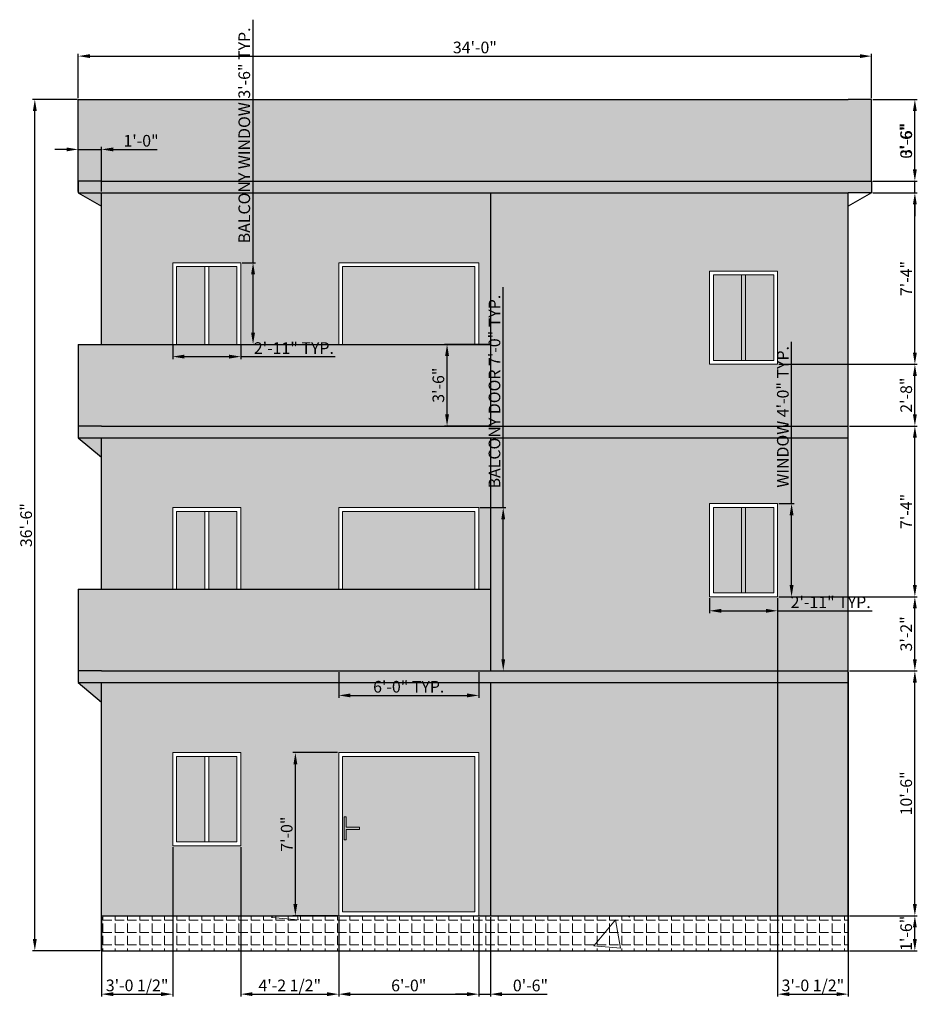
# Model space of a CAD drawing. Units: inches. Extents: x 2129 to 3258, y 1851 to 3021.
# Tile 10 of 10: x 2144 to 2605, y 2514 to 3021. Entities that reach past the tile are written whole.
import ezdxf

# ---------------------------------------------------------------- set-up
doc = ezdxf.new("R2010")
doc.units = ezdxf.units.IN
for name, color, linetype, lineweight in [('A-ANNO-DIMS', 2, 'Continuous', 18), ('A-ELEV', 7, 'Continuous', 25), ('A-ELEV-DOOR', 4, 'Continuous', 18), ('A-ELEV-DOOR-PATT', 34, 'Continuous', 13), ('A-ELEV-GLAZ', 4, 'Continuous', 18), ('A-ELEV-MASN-PATT', 7, 'Continuous', 13)]:
    doc.layers.add(name, color=color, linetype=linetype, lineweight=lineweight)
for name, color, linetype, lineweight, true_color in [('A-ELEV-BASE-PATT', 244, 'Continuous', 13, 0x991b1e), ('A-ELEV-GLAZ-PATT', 143, 'Continuous', 13, 0x7aafdf), ('A-ELEV-HDWR-PATT', 51, 'Continuous', 13, 0xf8f6b0), ('A-ELEV-TRIM-PATT', 244, 'Continuous', 13, 0x991b1e), ('A-ELEV-WALL-PATT', 116, 'Continuous', 13, 0x136734)]:
    doc.layers.add(name, color=color, linetype=linetype, lineweight=lineweight, true_color=true_color)
doc.styles.get("Standard").update_dxf_attribs({"font": 'arial.ttf'})
doc.dimstyles.new('ISO-25', dxfattribs={"dimtxt": 6, "dimasz": 6, "dimexe": 1.25, "dimexo": 0.625, "dimtad": 1, "dimdec": 1, "dimlunit": 3, "dimtxsty": 'Standard', "dimcen": 2.5, "dimclrd": 5, "dimclre": 5, "dimadec": 0, "dimazin": 0, "dimtfac": 1, "dimtdec": 1, "dimtmove": 0, "dimatfit": 3, "dimfxl": 1, "dimarcsym": 0})

# ---------------------------------------------------------------- blocks, each defined once
blk = doc.blocks.new('WIN-ELEV-35X48')
for p, q in [((16.5, 46), (16.5, 2)), ((18.5, 46), (18.5, 2))]:
    blk.add_line(p, q)
for points in [[(0, 0), (35, 0), (35, 48), (0, 48)], [(0, 0), (35, 0), (35, 48), (0, 48)], [(2, 2), (33, 2), (33, 46), (2, 46)]]:
    blk.add_lwpolyline(points, close=True)
blk = doc.blocks.new('WIN-ELEV-BALCONY')
for p, q in [((16.5, 40), (16.5, 0)), ((18.5, 40), (18.5, 0))]:
    blk.add_line(p, q)
for points in [[(35, 0), (35, 42), (0, 42), (0, 0)], [(35, 0), (35, 42), (0, 42), (0, 0)], [(33, 0), (33, 40), (2, 40), (2, 0)]]:
    blk.add_lwpolyline(points)
blk = doc.blocks.new('DOOR-ELEV-BALCONY')
for points in [[(72, 42), (72, 84), (0, 84), (0, 42)], [(72, 42), (72, 84), (0, 84), (0, 42)], [(70, 42), (70, 82), (2, 82), (2, 42)], [(0, 0), (72, 0)], [(0, 0), (72, 0)]]:
    blk.add_lwpolyline(points)
blk = doc.blocks.new('*D80')
at = {"layer": 'A-ANNO-DIMS', "color": 5, "lineweight": -2, "transparency": 16777216}
for p, q in [((2540.83, 2772.1), (2540.83, 2855.28)), ((2534.25, 2772.1), (2542.08, 2772.1)), ((2540.83, 2730.1), (2540.83, 2766.1)), ((2534.25, 2724.1), (2542.08, 2724.1))]:
    blk.add_line(p, q, dxfattribs=at)
at = {"layer": 'A-ANNO-DIMS', "color": 5, "transparency": 16777216}
for points in [[(2539.83, 2766.1), (2541.83, 2766.1), (2540.83, 2772.1)], [(2539.83, 2730.1), (2541.83, 2730.1), (2540.83, 2724.1)]]:
    blk.add_solid(points, dxfattribs=at)
at = {"layer": 'Defpoints', "color": 0, "transparency": 16777216}
for p in [(2533.63, 2772.1), (2540.83, 2772.1), (2533.63, 2724.1)]:
    blk.add_point(p, dxfattribs=at)
at = {"layer": 'A-ANNO-DIMS', "color": 0, "transparency": 16777216, "insert": (2537.1, 2816.69), "char_height": 6, "attachment_point": 5, "rotation": 90}
blk.add_mtext('WINDOW 4\'-0" TYP.', dxfattribs=at)
blk = doc.blocks.new('*D81')
at = {"layer": 'A-ANNO-DIMS', "color": 5, "lineweight": -2, "transparency": 16777216}
for p, q in [((2498.63, 2723.48), (2498.63, 2715.65)), ((2533.63, 2723.48), (2533.63, 2715.65)), ((2504.63, 2716.9), (2527.63, 2716.9)), ((2533.63, 2716.9), (2582.21, 2716.9))]:
    blk.add_line(p, q, dxfattribs=at)
at = {"layer": 'A-ANNO-DIMS', "color": 5, "transparency": 16777216}
for points in [[(2504.63, 2717.9), (2504.63, 2715.9), (2498.63, 2716.9)], [(2527.63, 2717.9), (2527.63, 2715.9), (2533.63, 2716.9)]]:
    blk.add_solid(points, dxfattribs=at)
at = {"layer": 'Defpoints', "color": 0, "transparency": 16777216}
for p in [(2498.63, 2724.1), (2533.63, 2724.1), (2533.63, 2716.9)]:
    blk.add_point(p, dxfattribs=at)
at = {"layer": 'A-ANNO-DIMS', "color": 0, "transparency": 16777216, "insert": (2560.92, 2720.54), "char_height": 6, "attachment_point": 5}
blk.add_mtext('2\'-11" TYP.', dxfattribs=at)
blk = doc.blocks.new('*D82')
at = {"layer": 'A-ANNO-DIMS', "color": 5, "lineweight": -2, "transparency": 16777216}
for p, q in [((2263.86, 2895.97), (2263.86, 3021.02)), ((2258.19, 2895.97), (2265.11, 2895.97)), ((2263.86, 2859.97), (2263.86, 2889.97)), ((2258.19, 2853.97), (2265.11, 2853.97))]:
    blk.add_line(p, q, dxfattribs=at)
at = {"layer": 'A-ANNO-DIMS', "color": 5, "transparency": 16777216}
for points in [[(2262.86, 2889.97), (2264.86, 2889.97), (2263.86, 2895.97)], [(2262.86, 2859.97), (2264.86, 2859.97), (2263.86, 2853.97)]]:
    blk.add_solid(points, dxfattribs=at)
at = {"layer": 'Defpoints', "color": 0, "transparency": 16777216}
for p in [(2257.56, 2895.97), (2263.86, 2895.97), (2257.56, 2853.97)]:
    blk.add_point(p, dxfattribs=at)
at = {"layer": 'A-ANNO-DIMS', "color": 0, "transparency": 16777216, "insert": (2260.13, 2961.49), "char_height": 6, "attachment_point": 5, "rotation": 90}
blk.add_mtext('BALCONY WINDOW 3\'-6" TYP.', dxfattribs=at)
blk = doc.blocks.new('*D83')
at = {"layer": 'A-ANNO-DIMS', "color": 5, "lineweight": -2, "transparency": 16777216}
for p, q in [((2222.56, 2853.34), (2222.56, 2846.42)), ((2257.56, 2853.34), (2257.56, 2846.42)), ((2228.56, 2847.67), (2251.56, 2847.67)), ((2257.56, 2847.67), (2306.15, 2847.67))]:
    blk.add_line(p, q, dxfattribs=at)
at = {"layer": 'A-ANNO-DIMS', "color": 5, "transparency": 16777216}
for points in [[(2228.56, 2848.67), (2228.56, 2846.67), (2222.56, 2847.67)], [(2251.56, 2848.67), (2251.56, 2846.67), (2257.56, 2847.67)]]:
    blk.add_solid(points, dxfattribs=at)
at = {"layer": 'Defpoints', "color": 0, "transparency": 16777216}
for p in [(2222.56, 2853.97), (2257.56, 2853.97), (2257.56, 2847.67)]:
    blk.add_point(p, dxfattribs=at)
at = {"layer": 'A-ANNO-DIMS', "color": 0, "transparency": 16777216, "insert": (2284.86, 2851.3), "char_height": 6, "attachment_point": 5}
blk.add_mtext('2\'-11" TYP.', dxfattribs=at)
blk = doc.blocks.new('*D84')
at = {"layer": 'A-ANNO-DIMS', "color": 5, "lineweight": -2, "transparency": 16777216}
for p, q in [((2392.53, 2769.97), (2392.53, 2883.39)), ((2380.55, 2769.97), (2393.78, 2769.97)), ((2392.53, 2691.97), (2392.53, 2763.97)), ((2380.55, 2685.97), (2393.78, 2685.97))]:
    blk.add_line(p, q, dxfattribs=at)
at = {"layer": 'A-ANNO-DIMS', "color": 5, "transparency": 16777216}
for points in [[(2391.53, 2763.97), (2393.53, 2763.97), (2392.53, 2769.97)], [(2391.53, 2691.97), (2393.53, 2691.97), (2392.53, 2685.97)]]:
    blk.add_solid(points, dxfattribs=at)
at = {"layer": 'Defpoints', "color": 0, "transparency": 16777216}
for p in [(2379.93, 2769.97), (2392.53, 2769.97), (2379.93, 2685.97)]:
    blk.add_point(p, dxfattribs=at)
at = {"layer": 'A-ANNO-DIMS', "color": 0, "transparency": 16777216, "insert": (2388.8, 2829.68), "char_height": 6, "attachment_point": 5, "rotation": 90}
blk.add_mtext('BALCONY DOOR 7\'-0" TYP.', dxfattribs=at)
blk = doc.blocks.new('*D85')
at = {"layer": 'A-ANNO-DIMS', "color": 5, "lineweight": -2, "transparency": 16777216}
for p, q in [((2307.93, 2685.34), (2307.93, 2672.12)), ((2379.93, 2685.34), (2379.93, 2672.12)), ((2313.93, 2673.37), (2373.93, 2673.37))]:
    blk.add_line(p, q, dxfattribs=at)
at = {"layer": 'A-ANNO-DIMS', "color": 5, "transparency": 16777216}
for points in [[(2313.93, 2674.37), (2313.93, 2672.37), (2307.93, 2673.37)], [(2373.93, 2674.37), (2373.93, 2672.37), (2379.93, 2673.37)]]:
    blk.add_solid(points, dxfattribs=at)
at = {"layer": 'Defpoints', "color": 0, "transparency": 16777216}
for p in [(2307.93, 2685.97), (2379.93, 2685.97), (2379.93, 2673.37)]:
    blk.add_point(p, dxfattribs=at)
at = {"layer": 'A-ANNO-DIMS', "color": 0, "transparency": 16777216, "insert": (2343.93, 2677.05), "char_height": 6, "attachment_point": 5}
blk.add_mtext('6\'-0" TYP.', dxfattribs=at)
blk = doc.blocks.new('*D115')
at = {"layer": 'A-ANNO-DIMS', "color": 5, "lineweight": -2, "transparency": 16777216}
for p, q in [((2173.98, 2980.59), (2173.98, 3003.52)), ((2179.98, 3002.27), (2575.93, 3002.27)), ((2581.93, 2980.59), (2581.93, 3003.52))]:
    blk.add_line(p, q, dxfattribs=at)
at = {"layer": 'A-ANNO-DIMS', "color": 5, "transparency": 16777216}
for points in [[(2179.98, 3003.27), (2179.98, 3001.27), (2173.98, 3002.27)], [(2575.93, 3003.27), (2575.93, 3001.27), (2581.93, 3002.27)]]:
    blk.add_solid(points, dxfattribs=at)
at = {"layer": 'Defpoints', "color": 0, "transparency": 16777216}
for p in [(2581.93, 3002.27), (2173.98, 2979.97), (2581.93, 2979.97)]:
    blk.add_point(p, dxfattribs=at)
at = {"layer": 'A-ANNO-DIMS', "color": 0, "transparency": 16777216, "insert": (2377.95, 3005.96), "char_height": 6, "attachment_point": 5}
blk.add_mtext('34\'-0"', dxfattribs=at)
blk = doc.blocks.new('*D116')
at = {"layer": 'A-ANNO-DIMS', "color": 5, "lineweight": -2, "transparency": 16777216}
for p, q in [((2173.35, 2979.97), (2150.38, 2979.97)), ((2151.63, 2547.97), (2151.63, 2973.97)), ((2185.3, 2541.97), (2150.38, 2541.97))]:
    blk.add_line(p, q, dxfattribs=at)
at = {"layer": 'A-ANNO-DIMS', "color": 5, "transparency": 16777216}
for points in [[(2150.63, 2973.97), (2152.63, 2973.97), (2151.63, 2979.97)], [(2150.63, 2547.97), (2152.63, 2547.97), (2151.63, 2541.97)]]:
    blk.add_solid(points, dxfattribs=at)
at = {"layer": 'Defpoints', "color": 0, "transparency": 16777216}
for p in [(2151.63, 2979.97), (2173.98, 2979.97), (2185.93, 2541.97)]:
    blk.add_point(p, dxfattribs=at)
at = {"layer": 'A-ANNO-DIMS', "color": 0, "transparency": 16777216, "insert": (2147.94, 2760.97), "char_height": 6, "attachment_point": 5, "rotation": 90}
blk.add_mtext('36\'-6"', dxfattribs=at)
blk = doc.blocks.new('*D117')
at = {"layer": 'A-ANNO-DIMS', "color": 5, "lineweight": -2, "transparency": 16777216}
for p, q in [((2570.55, 2559.97), (2605.48, 2559.97)), ((2604.23, 2547.97), (2604.23, 2553.97)), ((2570.55, 2541.97), (2605.48, 2541.97))]:
    blk.add_line(p, q, dxfattribs=at)
at = {"layer": 'A-ANNO-DIMS', "color": 5, "transparency": 16777216}
for points in [[(2603.23, 2553.97), (2605.23, 2553.97), (2604.23, 2559.97)], [(2603.23, 2547.97), (2605.23, 2547.97), (2604.23, 2541.97)]]:
    blk.add_solid(points, dxfattribs=at)
at = {"layer": 'Defpoints', "color": 0, "transparency": 16777216}
for p in [(2569.93, 2559.97), (2604.23, 2559.97), (2569.93, 2541.97)]:
    blk.add_point(p, dxfattribs=at)
at = {"layer": 'A-ANNO-DIMS', "color": 0, "transparency": 16777216, "insert": (2600.54, 2550.97), "char_height": 6, "attachment_point": 5, "rotation": 90}
blk.add_mtext('1\'-6"', dxfattribs=at)
blk = doc.blocks.new('*D118')
at = {"layer": 'A-ANNO-DIMS', "color": 5, "lineweight": -2, "transparency": 16777216}
for p, q in [((2570.55, 2685.97), (2605.48, 2685.97)), ((2604.23, 2565.97), (2604.23, 2679.97)), ((2570.55, 2559.97), (2605.48, 2559.97))]:
    blk.add_line(p, q, dxfattribs=at)
at = {"layer": 'A-ANNO-DIMS', "color": 5, "transparency": 16777216}
for points in [[(2603.23, 2679.97), (2605.23, 2679.97), (2604.23, 2685.97)], [(2603.23, 2565.97), (2605.23, 2565.97), (2604.23, 2559.97)]]:
    blk.add_solid(points, dxfattribs=at)
at = {"layer": 'Defpoints', "color": 0, "transparency": 16777216}
for p in [(2569.93, 2685.97), (2604.23, 2685.97), (2569.93, 2559.97)]:
    blk.add_point(p, dxfattribs=at)
at = {"layer": 'A-ANNO-DIMS', "color": 0, "transparency": 16777216, "insert": (2600.54, 2622.97), "char_height": 6, "attachment_point": 5, "rotation": 90}
blk.add_mtext('10\'-6"', dxfattribs=at)
blk = doc.blocks.new('*D119')
at = {"layer": 'A-ANNO-DIMS', "color": 5, "lineweight": -2, "transparency": 16777216}
for p, q in [((2534.25, 2724.1), (2605.48, 2724.1)), ((2604.23, 2691.97), (2604.23, 2718.1)), ((2570.55, 2685.97), (2605.48, 2685.97))]:
    blk.add_line(p, q, dxfattribs=at)
at = {"layer": 'A-ANNO-DIMS', "color": 5, "transparency": 16777216}
for points in [[(2603.23, 2718.1), (2605.23, 2718.1), (2604.23, 2724.1)], [(2603.23, 2691.97), (2605.23, 2691.97), (2604.23, 2685.97)]]:
    blk.add_solid(points, dxfattribs=at)
at = {"layer": 'Defpoints', "color": 0, "transparency": 16777216}
for p in [(2533.63, 2724.1), (2604.23, 2724.1), (2569.93, 2685.97)]:
    blk.add_point(p, dxfattribs=at)
at = {"layer": 'A-ANNO-DIMS', "color": 0, "transparency": 16777216, "insert": (2600.54, 2705.03), "char_height": 6, "attachment_point": 5, "rotation": 90}
blk.add_mtext('3\'-2"', dxfattribs=at)
blk = doc.blocks.new('*D120')
at = {"layer": 'A-ANNO-DIMS', "color": 5, "lineweight": -2, "transparency": 16777216}
for p, q in [((2570.552986, 2811.965219), (2605.477986, 2811.965219)), ((2604.227986, 2730.103007), (2604.227986, 2805.965219)), ((2534.252329, 2724.103007), (2605.477986, 2724.103007))]:
    blk.add_line(p, q, dxfattribs=at)
at = {"layer": 'A-ANNO-DIMS', "color": 5, "transparency": 16777216}
for points in [[(2603.227986, 2805.965219), (2605.227986, 2805.965219), (2604.227986, 2811.965219)], [(2603.227986, 2730.103007), (2605.227986, 2730.103007), (2604.227986, 2724.103007)]]:
    blk.add_solid(points, dxfattribs=at)
at = {"layer": 'Defpoints', "color": 0, "transparency": 16777216}
for p in [(2569.927986, 2811.965219), (2604.227986, 2811.965219), (2533.627329, 2724.103007)]:
    blk.add_point(p, dxfattribs=at)
at = {"layer": 'A-ANNO-DIMS', "color": 0, "transparency": 16777216, "insert": (2600.602986, 2768.034113), "char_height": 6, "attachment_point": 5, "rotation": 90}
blk.add_mtext('7\'-4"', dxfattribs=at)
blk = doc.blocks.new('*D121')
at = {"layer": 'A-ANNO-DIMS', "color": 5, "lineweight": -2, "transparency": 16777216}
for p, q in [((2534.25, 2843.72), (2605.48, 2843.72)), ((2604.23, 2817.97), (2604.23, 2837.72)), ((2570.55, 2811.97), (2605.48, 2811.97))]:
    blk.add_line(p, q, dxfattribs=at)
at = {"layer": 'A-ANNO-DIMS', "color": 5, "transparency": 16777216}
for points in [[(2603.23, 2837.72), (2605.23, 2837.72), (2604.23, 2843.72)], [(2603.23, 2817.97), (2605.23, 2817.97), (2604.23, 2811.97)]]:
    blk.add_solid(points, dxfattribs=at)
at = {"layer": 'Defpoints', "color": 0, "transparency": 16777216}
for p in [(2533.63, 2843.72), (2604.23, 2843.72), (2569.93, 2811.97)]:
    blk.add_point(p, dxfattribs=at)
at = {"layer": 'A-ANNO-DIMS', "color": 0, "transparency": 16777216, "insert": (2600.54, 2827.84), "char_height": 6, "attachment_point": 5, "rotation": 90}
blk.add_mtext('2\'-8"', dxfattribs=at)
blk = doc.blocks.new('*D122')
at = {"layer": 'A-ANNO-DIMS', "color": 5, "lineweight": -2, "transparency": 16777216}
for p, q in [((2582.552986, 2931.965219), (2605.477986, 2931.965219)), ((2604.227986, 2849.721947), (2604.227986, 2925.965219)), ((2534.252329, 2843.721947), (2605.477986, 2843.721947))]:
    blk.add_line(p, q, dxfattribs=at)
at = {"layer": 'A-ANNO-DIMS', "color": 5, "transparency": 16777216}
for points in [[(2603.227986, 2925.965219), (2605.227986, 2925.965219), (2604.227986, 2931.965219)], [(2603.227986, 2849.721947), (2605.227986, 2849.721947), (2604.227986, 2843.721947)]]:
    blk.add_solid(points, dxfattribs=at)
at = {"layer": 'Defpoints', "color": 0, "transparency": 16777216}
for p in [(2581.927986, 2931.965219), (2604.227986, 2931.965219), (2533.627329, 2843.721947)]:
    blk.add_point(p, dxfattribs=at)
at = {"layer": 'A-ANNO-DIMS', "color": 0, "transparency": 16777216, "insert": (2600.602986, 2887.843583), "char_height": 6, "attachment_point": 5, "rotation": 90}
blk.add_mtext('7\'-4"', dxfattribs=at)
blk = doc.blocks.new('*D123')
at = {"layer": 'A-ANNO-DIMS', "color": 5, "lineweight": -2, "transparency": 16777216}
for p, q in [((2604.23, 2943.97), (2604.23, 2967.16)), ((2582.55, 2937.97), (2605.48, 2937.97)), ((2604.23, 2931.97), (2604.23, 2937.97)), ((2582.55, 2931.97), (2605.48, 2931.97)), ((2604.23, 2925.97), (2604.23, 2919.97))]:
    blk.add_line(p, q, dxfattribs=at)
at = {"layer": 'A-ANNO-DIMS', "color": 5, "transparency": 16777216}
for points in [[(2603.23, 2943.97), (2605.23, 2943.97), (2604.23, 2937.97)], [(2603.23, 2925.97), (2605.23, 2925.97), (2604.23, 2931.97)]]:
    blk.add_solid(points, dxfattribs=at)
at = {"layer": 'Defpoints', "color": 0, "transparency": 16777216}
for p in [(2581.93, 2937.97), (2604.23, 2937.97), (2581.93, 2931.97)]:
    blk.add_point(p, dxfattribs=at)
at = {"layer": 'A-ANNO-DIMS', "color": 0, "transparency": 16777216, "insert": (2600.54, 2958.56), "char_height": 6, "attachment_point": 5, "rotation": 90}
blk.add_mtext('0\'-6"', dxfattribs=at)
blk = doc.blocks.new('*D124')
at = {"layer": 'A-ANNO-DIMS', "color": 5, "lineweight": -2, "transparency": 16777216}
for p, q in [((2582.55, 2979.97), (2605.48, 2979.97)), ((2604.23, 2943.97), (2604.23, 2973.97)), ((2582.55, 2937.97), (2605.48, 2937.97))]:
    blk.add_line(p, q, dxfattribs=at)
at = {"layer": 'A-ANNO-DIMS', "color": 5, "transparency": 16777216}
for points in [[(2603.23, 2973.97), (2605.23, 2973.97), (2604.23, 2979.97)], [(2603.23, 2943.97), (2605.23, 2943.97), (2604.23, 2937.97)]]:
    blk.add_solid(points, dxfattribs=at)
at = {"layer": 'Defpoints', "color": 0, "transparency": 16777216}
for p in [(2581.93, 2979.97), (2604.23, 2979.97), (2581.93, 2937.97)]:
    blk.add_point(p, dxfattribs=at)
at = {"layer": 'A-ANNO-DIMS', "color": 0, "transparency": 16777216, "insert": (2600.54, 2958.97), "char_height": 6, "attachment_point": 5, "rotation": 90}
blk.add_mtext('3\'-6"', dxfattribs=at)
blk = doc.blocks.new('*D125')
at = {"layer": 'A-ANNO-DIMS', "color": 5, "lineweight": -2, "transparency": 16777216}
for p, q in [((2222.56, 2595.34), (2222.56, 2518.42)), ((2185.93, 2559.34), (2185.93, 2518.42)), ((2191.93, 2519.67), (2216.56, 2519.67))]:
    blk.add_line(p, q, dxfattribs=at)
at = {"layer": 'A-ANNO-DIMS', "color": 5, "transparency": 16777216}
for points in [[(2191.93, 2520.67), (2191.93, 2518.67), (2185.93, 2519.67)], [(2216.56, 2520.67), (2216.56, 2518.67), (2222.56, 2519.67)]]:
    blk.add_solid(points, dxfattribs=at)
at = {"layer": 'Defpoints', "color": 0, "transparency": 16777216}
for p in [(2222.56, 2595.97), (2185.93, 2559.97), (2222.56, 2519.67)]:
    blk.add_point(p, dxfattribs=at)
at = {"layer": 'A-ANNO-DIMS', "color": 0, "transparency": 16777216, "insert": (2204.25, 2523.39), "char_height": 6, "attachment_point": 5}
blk.add_mtext('3\'-0 1/2"', dxfattribs=at)
blk = doc.blocks.new('*D126')
at = {"layer": 'A-ANNO-DIMS', "color": 5, "lineweight": -2, "transparency": 16777216}
for p, q in [((2257.56, 2595.34), (2257.56, 2518.42)), ((2307.93, 2559.34), (2307.93, 2518.42)), ((2263.56, 2519.67), (2301.93, 2519.67))]:
    blk.add_line(p, q, dxfattribs=at)
at = {"layer": 'A-ANNO-DIMS', "color": 5, "transparency": 16777216}
for points in [[(2263.56, 2520.67), (2263.56, 2518.67), (2257.56, 2519.67)], [(2301.93, 2520.67), (2301.93, 2518.67), (2307.93, 2519.67)]]:
    blk.add_solid(points, dxfattribs=at)
at = {"layer": 'Defpoints', "color": 0, "transparency": 16777216}
for p in [(2257.56, 2595.97), (2307.93, 2559.97), (2307.93, 2519.67)]:
    blk.add_point(p, dxfattribs=at)
at = {"layer": 'A-ANNO-DIMS', "color": 0, "transparency": 16777216, "insert": (2282.75, 2523.39), "char_height": 6, "attachment_point": 5}
blk.add_mtext('4\'-2 1/2"', dxfattribs=at)
blk = doc.blocks.new('*D127')
at = {"layer": 'A-ANNO-DIMS', "color": 5, "lineweight": -2, "transparency": 16777216}
for p, q in [((2379.93, 2559.34), (2379.93, 2518.42)), ((2385.93, 2559.34), (2385.93, 2518.42)), ((2373.93, 2519.67), (2367.93, 2519.67)), ((2379.93, 2519.67), (2385.93, 2519.67)), ((2391.93, 2519.67), (2415.13, 2519.67))]:
    blk.add_line(p, q, dxfattribs=at)
at = {"layer": 'A-ANNO-DIMS', "color": 5, "transparency": 16777216}
for points in [[(2373.93, 2520.67), (2373.93, 2518.67), (2379.93, 2519.67)], [(2391.93, 2520.67), (2391.93, 2518.67), (2385.93, 2519.67)]]:
    blk.add_solid(points, dxfattribs=at)
at = {"layer": 'Defpoints', "color": 0, "transparency": 16777216}
for p in [(2379.93, 2559.97), (2385.93, 2559.97), (2385.93, 2519.67)]:
    blk.add_point(p, dxfattribs=at)
at = {"layer": 'A-ANNO-DIMS', "color": 0, "transparency": 16777216, "insert": (2406.53, 2523.35), "char_height": 6, "attachment_point": 5}
blk.add_mtext('0\'-6"', dxfattribs=at)
blk = doc.blocks.new('*D128')
at = {"layer": 'A-ANNO-DIMS', "color": 5, "lineweight": -2, "transparency": 16777216}
for p, q in [((2533.63, 2723.48), (2533.63, 2518.42)), ((2569.93, 2685.34), (2569.93, 2518.42)), ((2539.63, 2519.67), (2563.93, 2519.67))]:
    blk.add_line(p, q, dxfattribs=at)
at = {"layer": 'A-ANNO-DIMS', "color": 5, "transparency": 16777216}
for points in [[(2539.63, 2520.67), (2539.63, 2518.67), (2533.63, 2519.67)], [(2563.93, 2520.67), (2563.93, 2518.67), (2569.93, 2519.67)]]:
    blk.add_solid(points, dxfattribs=at)
at = {"layer": 'Defpoints', "color": 0, "transparency": 16777216}
for p in [(2533.63, 2724.1), (2569.93, 2685.97), (2569.93, 2519.67)]:
    blk.add_point(p, dxfattribs=at)
at = {"layer": 'A-ANNO-DIMS', "color": 0, "transparency": 16777216, "insert": (2551.78, 2523.39), "char_height": 6, "attachment_point": 5}
blk.add_mtext('3\'-0 1/2"', dxfattribs=at)
blk = doc.blocks.new('*D129')
at = {"layer": 'A-ANNO-DIMS', "color": 5, "lineweight": -2, "transparency": 16777216}
for p, q in [((2307.3, 2643.97), (2284.38, 2643.97)), ((2285.63, 2565.97), (2285.63, 2637.97)), ((2307.3, 2559.97), (2284.38, 2559.97))]:
    blk.add_line(p, q, dxfattribs=at)
at = {"layer": 'A-ANNO-DIMS', "color": 5, "transparency": 16777216}
for points in [[(2284.63, 2637.97), (2286.63, 2637.97), (2285.63, 2643.97)], [(2284.63, 2565.97), (2286.63, 2565.97), (2285.63, 2559.97)]]:
    blk.add_solid(points, dxfattribs=at)
at = {"layer": 'Defpoints', "color": 0, "transparency": 16777216}
for p in [(2285.63, 2643.97), (2307.93, 2643.97), (2307.93, 2559.97)]:
    blk.add_point(p, dxfattribs=at)
at = {"layer": 'A-ANNO-DIMS', "color": 0, "transparency": 16777216, "insert": (2281.94, 2601.97), "char_height": 6, "attachment_point": 5, "rotation": 90}
blk.add_mtext('7\'-0"', dxfattribs=at)
blk = doc.blocks.new('*D130')
at = {"layer": 'A-ANNO-DIMS', "color": 5, "lineweight": -2, "transparency": 16777216}
for p, q in [((2385.3, 2853.97), (2362.38, 2853.97)), ((2363.63, 2817.97), (2363.63, 2847.97)), ((2385.3, 2811.97), (2362.38, 2811.97))]:
    blk.add_line(p, q, dxfattribs=at)
at = {"layer": 'A-ANNO-DIMS', "color": 5, "transparency": 16777216}
for points in [[(2362.63, 2847.97), (2364.63, 2847.97), (2363.63, 2853.97)], [(2362.63, 2817.97), (2364.63, 2817.97), (2363.63, 2811.97)]]:
    blk.add_solid(points, dxfattribs=at)
at = {"layer": 'Defpoints', "color": 0, "transparency": 16777216}
for p in [(2363.63, 2853.97), (2385.93, 2853.97), (2385.93, 2811.97)]:
    blk.add_point(p, dxfattribs=at)
at = {"layer": 'A-ANNO-DIMS', "color": 0, "transparency": 16777216, "insert": (2359.94, 2832.97), "char_height": 6, "attachment_point": 5, "rotation": 90}
blk.add_mtext('3\'-6"', dxfattribs=at)
blk = doc.blocks.new('*D131')
at = {"layer": 'A-ANNO-DIMS', "color": 5, "lineweight": -2, "transparency": 16777216}
for p, q in [((2307.93, 2559.34), (2307.93, 2518.42)), ((2379.93, 2559.34), (2379.93, 2518.42)), ((2313.93, 2519.67), (2373.93, 2519.67))]:
    blk.add_line(p, q, dxfattribs=at)
at = {"layer": 'A-ANNO-DIMS', "color": 5, "transparency": 16777216}
for points in [[(2313.93, 2520.67), (2313.93, 2518.67), (2307.93, 2519.67)], [(2373.93, 2520.67), (2373.93, 2518.67), (2379.93, 2519.67)]]:
    blk.add_solid(points, dxfattribs=at)
at = {"layer": 'Defpoints', "color": 0, "transparency": 16777216}
for p in [(2307.93, 2559.97), (2379.93, 2559.97), (2379.93, 2519.67)]:
    blk.add_point(p, dxfattribs=at)
at = {"layer": 'A-ANNO-DIMS', "color": 0, "transparency": 16777216, "insert": (2343.93, 2523.35), "char_height": 6, "attachment_point": 5}
blk.add_mtext('6\'-0"', dxfattribs=at)
blk = doc.blocks.new('*D132')
at = {"layer": 'A-ANNO-DIMS', "color": 5, "lineweight": -2, "transparency": 16777216}
for p, q in [((2167.93, 2954.27), (2161.93, 2954.27)), ((2173.93, 2932.59), (2173.93, 2955.52)), ((2173.93, 2954.27), (2185.93, 2954.27)), ((2185.93, 2932.59), (2185.93, 2955.52)), ((2191.93, 2954.27), (2214.56, 2954.27))]:
    blk.add_line(p, q, dxfattribs=at)
at = {"layer": 'A-ANNO-DIMS', "color": 5, "transparency": 16777216}
for points in [[(2167.93, 2955.27), (2167.93, 2953.27), (2173.93, 2954.27)], [(2191.93, 2955.27), (2191.93, 2953.27), (2185.93, 2954.27)]]:
    blk.add_solid(points, dxfattribs=at)
at = {"layer": 'Defpoints', "color": 0, "transparency": 16777216}
for p in [(2185.93, 2954.27), (2173.93, 2931.97), (2185.93, 2931.97)]:
    blk.add_point(p, dxfattribs=at)
at = {"layer": 'A-ANNO-DIMS', "color": 0, "transparency": 16777216, "insert": (2206.25, 2957.95), "char_height": 6, "attachment_point": 5}
blk.add_mtext('1\'-0"', dxfattribs=at)

msp = doc.modelspace()

# ---------------------------------------------------------------- hatches: boundary and pattern name
at = {"layer": 'A-ELEV-BASE-PATT', "transparency": 33554585}
h = msp.add_hatch(dxfattribs=at)
h.set_pattern_fill('AR-CONC', color=256, scale=0.91)
h.set_pattern_definition([(50, (0, -150.12), (165.788, -14.5046), [17.3355, -190.6905]), (355, (0, -150.12), (-32.0715, 173.862), [13.8684, -152.553]), (100.4514, (13.82, -151.33), (133.7165, 159.357), [14.733, -162.062]), (46.184, (0, -103.9), (246.682, -38.259), [26.003, -286.036]), (96.6356, (20.56, -107.08), (216.038, 225.158), [22.1, -243.093]), (351.184, (0, -103.9), (216.038, 225.158), [20.803, -228.828]), (21, (23.11, -115.45), (137.969, -93.0613), [17.3355, -190.6905]), (326, (23.11, -115.45), (56.24, 167.611), [13.8684, -152.5524]), (71.4514, (34.61, -123.21), (194.209, 74.55), [14.733, -162.062]), (37.5, (0, -150.125), (2.8106, 76.9451), [0, -150.7033, 0, -154.8638, 0, -153.1302]), (7.5, (0, -150.125), (60.8059, 91.1643), [0, -88.2955, 0, -147.2362, 0, -58.3629]), (327.5, (-51.544, -150.125), (123.3874, -5.2132), [0, -57.785, 0, -180.2892, 0, -239.23]), (317.5, (-74.66, -150.12), (134.7976, 23.138), [0, -75.1205, 0, -119.7305, 0, -169.888])])
h.paths.add_polyline_path([(2569.93, 2559.97), (2185.93, 2559.97), (2185.93, 2541.97), (2569.93, 2541.97)])
at = {"layer": 'A-ELEV-DOOR-PATT', "transparency": 33554658}
h = msp.add_hatch(color=256, dxfattribs=at)
h.dxf.hatch_style = 1
h.paths.add_polyline_path([(2377.93, 2767.97), (2309.93, 2767.97), (2309.93, 2727.97), (2377.93, 2727.97)])
h.paths.add_polyline_path([(2377.93, 2893.97), (2309.93, 2893.97), (2309.93, 2853.97), (2377.93, 2853.97)])
h = msp.add_hatch(color=256, dxfattribs=at)
h.dxf.hatch_style = 1
h.paths.add_polyline_path([(2377.93, 2641.97), (2309.93, 2641.97), (2309.93, 2561.97), (2377.93, 2561.97)])
at = {"layer": 'A-ELEV-GLAZ-PATT', "transparency": 33554658}
h = msp.add_hatch(color=256, dxfattribs=at)
h.dxf.hatch_style = 1
h.paths.add_polyline_path([(2239.06, 2641.97), (2224.56, 2641.97), (2224.56, 2597.97), (2239.06, 2597.97)])
h.paths.add_polyline_path([(2255.56, 2641.97), (2241.06, 2641.97), (2241.06, 2597.97), (2255.56, 2597.97)])
h.paths.add_polyline_path([(2239.06, 2767.97), (2224.56, 2767.97), (2224.56, 2727.97), (2239.06, 2727.97)])
h.paths.add_polyline_path([(2255.56, 2767.97), (2241.06, 2767.97), (2241.06, 2727.97), (2255.56, 2727.97)])
h.paths.add_polyline_path([(2239.06, 2893.97), (2224.56, 2893.97), (2224.56, 2853.97), (2239.06, 2853.97)])
h.paths.add_polyline_path([(2255.56, 2893.97), (2241.06, 2893.97), (2241.06, 2853.97), (2255.56, 2853.97)])
h.paths.add_polyline_path([(2515.13, 2889.72), (2500.63, 2889.72), (2500.63, 2845.72), (2515.13, 2845.72)])
h.paths.add_polyline_path([(2531.63, 2889.72), (2515.13, 2889.72), (2515.13, 2845.72), (2531.63, 2845.72)])
h.paths.add_polyline_path([(2515.13, 2770.1), (2500.63, 2770.1), (2500.63, 2726.1), (2515.13, 2726.1)])
h.paths.add_polyline_path([(2531.63, 2770.1), (2515.13, 2770.1), (2515.13, 2726.1), (2531.63, 2726.1)])
at = {"layer": 'A-ELEV-HDWR-PATT', "transparency": 33554585}
h = msp.add_hatch(color=256, dxfattribs=at)
h.dxf.hatch_style = 1
h.paths.add_polyline_path([(2311.75, 2604.38), (2318.56, 2604.38), (2318.56, 2605.59), (2311.75, 2605.59), (2311.75, 2610.87), (2310.78, 2610.87), (2310.78, 2598.98), (2311.75, 2598.98)])
at = {"layer": 'A-ELEV-MASN-PATT', "transparency": 33554585}
h = msp.add_hatch(dxfattribs=at)
h.set_pattern_fill('ANGLE', color=256, scale=0.91)
h.set_pattern_definition([(0, (0, -150.1245), (0, 6.35635), [4.6228, -1.73355]), (90, (0, -150.1245), (-6.35635, 4e-16), [4.6228, -1.73355])])
h.paths.add_polyline_path([(2569.93, 2559.97), (2185.93, 2559.97), (2185.93, 2541.97), (2569.93, 2541.97)])
at = {"layer": 'A-ELEV-TRIM-PATT', "transparency": 33554585}
h = msp.add_hatch(color=256, dxfattribs=at)
h.dxf.hatch_style = 1
h.paths.add_polyline_path([(2581.93, 2979.97), (2569.93, 2979.97), (2185.93, 2979.97), (2173.98, 2979.97), (2173.98, 2937.97), (2185.93, 2937.97), (2569.93, 2937.97), (2581.93, 2937.97)])
h = msp.add_hatch(color=256, dxfattribs=at)
h.dxf.hatch_style = 1
h.paths.add_polyline_path([(2581.93, 2937.97), (2569.93, 2937.97), (2185.93, 2937.97), (2173.93, 2937.97), (2173.93, 2931.97), (2185.93, 2931.97), (2569.93, 2931.97), (2581.93, 2931.97)])
h = msp.add_hatch(color=256, dxfattribs=at)
h.dxf.hatch_style = 1
h.paths.add_polyline_path([(2185.93, 2931.97), (2173.93, 2931.97), (2185.93, 2925.04)])
h = msp.add_hatch(color=256, dxfattribs=at)
h.dxf.hatch_style = 1
h.paths.add_polyline_path([(2385.93, 2853.97), (2173.93, 2853.97), (2173.93, 2811.97), (2185.93, 2811.97), (2385.93, 2811.97)])
h.paths.add_polyline_path([(2385.93, 2727.97), (2173.93, 2727.97), (2173.93, 2685.97), (2185.93, 2685.97), (2385.93, 2685.97)])
h = msp.add_hatch(color=256, dxfattribs=at)
h.dxf.hatch_style = 1
h.paths.add_polyline_path([(2569.93, 2811.97), (2185.93, 2811.97), (2173.93, 2811.97), (2173.93, 2805.97), (2185.93, 2805.97), (2569.93, 2805.97)])
h.paths.add_polyline_path([(2185.93, 2805.97), (2173.93, 2805.97), (2185.93, 2795.9)])
h.paths.add_polyline_path([(2569.93, 2685.97), (2185.93, 2685.97), (2173.93, 2685.97), (2173.93, 2679.97), (2185.93, 2679.97), (2569.93, 2679.97)])
h.paths.add_polyline_path([(2185.93, 2679.97), (2173.93, 2679.97), (2185.93, 2669.9)])
at = {"layer": 'A-ELEV-WALL-PATT', "transparency": 33554585}
h = msp.add_hatch(color=256, dxfattribs=at)
h.dxf.hatch_style = 1
h.paths.add_polyline_path([(2385.93, 2931.97), (2185.93, 2931.97), (2185.93, 2853.97), (2222.56, 2853.97), (2222.56, 2895.97), (2257.56, 2895.97), (2257.56, 2853.97), (2307.93, 2853.97), (2307.93, 2895.97), (2379.93, 2895.97), (2379.93, 2853.97), (2385.93, 2853.97)])
h.paths.add_polyline_path([(2569.93, 2931.97), (2385.93, 2931.97), (2385.93, 2853.97), (2385.93, 2811.97), (2569.93, 2811.97)])
h.paths.add_polyline_path([(2498.63, 2891.72), (2533.63, 2891.72), (2533.63, 2843.72), (2498.63, 2843.72)], flags=16)
h.paths.add_polyline_path([(2500.63, 2889.72), (2531.63, 2889.72), (2531.63, 2845.72), (2500.63, 2845.72)], flags=0)
h.paths.add_polyline_path([(2569.93, 2805.97), (2385.93, 2805.97), (2385.93, 2685.97), (2569.93, 2685.97)])
h.paths.add_polyline_path([(2498.63, 2772.1), (2533.63, 2772.1), (2533.63, 2724.1), (2498.63, 2724.1)], flags=16)
h.paths.add_polyline_path([(2500.63, 2770.1), (2531.63, 2770.1), (2531.63, 2726.1), (2500.63, 2726.1)], flags=0)
h.paths.add_polyline_path([(2569.93, 2679.97), (2385.93, 2679.97), (2385.93, 2559.97), (2569.93, 2559.97)])
h.paths.add_polyline_path([(2385.93, 2679.97), (2185.93, 2679.97), (2185.93, 2667.97), (2185.93, 2559.97), (2307.93, 2559.97), (2307.93, 2643.97), (2379.93, 2643.97), (2379.93, 2559.97), (2385.93, 2559.97)])
h.paths.add_polyline_path([(2257.56, 2643.97), (2257.56, 2595.97), (2222.56, 2595.97), (2222.56, 2643.97)], flags=16)
h.paths.add_polyline_path([(2255.56, 2641.97), (2255.56, 2597.97), (2224.56, 2597.97), (2224.56, 2641.97)], flags=0)
h.paths.add_polyline_path([(2385.93, 2805.97), (2185.93, 2805.97), (2185.93, 2727.97), (2222.56, 2727.97), (2222.56, 2769.97), (2257.56, 2769.97), (2257.56, 2727.97), (2307.93, 2727.97), (2307.93, 2769.97), (2379.93, 2769.97), (2379.93, 2727.97), (2385.93, 2727.97)])

# ---------------------------------------------------------------- linework, layer by layer
at = {"layer": 'A-ELEV'}
for p, q in [((2173.98, 2937.97), (2173.98, 2979.97)), ((2173.98, 2979.97), (2185.93, 2979.97)), ((2185.93, 2979.97), (2569.93, 2979.97)), ((2581.93, 2979.97), (2569.93, 2979.97)), ((2581.93, 2937.97), (2581.93, 2979.97)), ((2185.93, 2937.97), (2173.93, 2937.97)), ((2173.93, 2937.97), (2173.93, 2931.97)), ((2185.93, 2937.97), (2569.93, 2937.97)), ((2569.93, 2937.97), (2581.93, 2937.97)), ((2581.93, 2937.97), (2581.93, 2931.97)), ((2173.93, 2931.97), (2185.93, 2931.97)), ((2173.93, 2931.97), (2185.93, 2925.04)), ((2185.93, 2931.97), (2569.93, 2931.97)), ((2185.93, 2853.97), (2185.93, 2931.97)), ((2385.93, 2931.97), (2385.93, 2811.97)), ((2581.93, 2931.97), (2569.93, 2931.97)), ((2569.93, 2805.97), (2569.93, 2931.97)), ((2581.93, 2931.97), (2569.93, 2925.04)), ((2173.93, 2853.97), (2385.93, 2853.97)), ((2173.93, 2853.97), (2173.93, 2805.97)), ((2569.93, 2811.97), (2569.93, 2853.97)), ((2185.93, 2811.97), (2173.93, 2811.97)), ((2173.93, 2811.97), (2173.93, 2805.97)), ((2185.93, 2811.97), (2569.93, 2811.97)), ((2185.93, 2811.97), (2569.93, 2811.97)), ((2173.93, 2805.97), (2185.93, 2805.97)), ((2173.93, 2805.97), (2185.93, 2805.97)), ((2173.93, 2805.97), (2185.93, 2795.9)), ((2185.93, 2805.97), (2569.93, 2805.97)), ((2185.93, 2727.97), (2185.93, 2805.97)), ((2385.93, 2805.97), (2385.93, 2685.97)), ((2569.93, 2793.97), (2569.93, 2805.97)), ((2569.93, 2679.97), (2569.93, 2805.97)), ((2173.93, 2727.97), (2385.93, 2727.97)), ((2173.93, 2727.97), (2173.93, 2685.97)), ((2569.93, 2679.97), (2569.93, 2727.97)), ((2185.93, 2685.97), (2173.93, 2685.97)), ((2173.93, 2685.97), (2173.93, 2679.97)), ((2185.93, 2685.97), (2569.93, 2685.97)), ((2185.93, 2685.97), (2569.93, 2685.97)), ((2173.93, 2679.97), (2185.93, 2679.97)), ((2173.93, 2679.97), (2185.93, 2669.9)), ((2185.93, 2679.97), (2569.93, 2679.97)), ((2185.93, 2541.97), (2185.93, 2679.97)), ((2185.93, 2667.97), (2185.93, 2679.97)), ((2185.93, 2679.97), (2569.93, 2679.97)), ((2385.93, 2679.97), (2385.93, 2559.97)), ((2569.93, 2541.97), (2569.93, 2679.97)), ((2569.93, 2667.97), (2569.93, 2679.97)), ((2185.93, 2559.97), (2569.93, 2559.97)), ((2185.93, 2541.97), (2569.93, 2541.97))]:
    msp.add_line(p, q, dxfattribs=at)
at = {"layer": 'A-ELEV-DOOR'}
for points in [[(2307.93, 2559.97), (2379.93, 2559.97), (2379.93, 2643.97), (2307.93, 2643.97)], [(2307.93, 2559.97), (2379.93, 2559.97), (2379.93, 2643.97), (2307.93, 2643.97)], [(2309.93, 2561.97), (2377.93, 2561.97), (2377.93, 2641.97), (2309.93, 2641.97)]]:
    msp.add_lwpolyline(points, close=True, dxfattribs=at)
for points in [[(2311.75, 2605.59), (2311.75, 2610.87), (2310.78, 2610.87), (2310.78, 2598.98), (2311.75, 2598.98), (2311.75, 2604.38)], [(2310.78, 2604.38), (2310.78, 2605.59)], [(2311.75, 2605.59), (2318.56, 2605.59), (2318.56, 2604.38), (2311.75, 2604.38)]]:
    msp.add_lwpolyline(points, dxfattribs=at)

# ---------------------------------------------------------------- block references
for p in [(2307.93, 2811.97), (2307.93, 2685.97)]:
    msp.add_blockref('DOOR-ELEV-BALCONY', p, dxfattribs=at)
at = {"layer": 'A-ELEV-GLAZ'}
for name, p in [('WIN-ELEV-BALCONY', (2222.56, 2853.97)), ('WIN-ELEV-35X48', (2498.63, 2843.72)), ('WIN-ELEV-35X48', (2498.63, 2724.1)), ('WIN-ELEV-BALCONY', (2222.56, 2727.97)), ('WIN-ELEV-35X48', (2222.56, 2595.97))]:
    msp.add_blockref(name, p, dxfattribs=at)

# ---------------------------------------------------------------- dimensions: what is measured, and where the dimension line sits
at = {"layer": 'A-ANNO-DIMS'}
for base, p1, p2, text, picture, middle in [((2263.86, 2895.97), (2257.56, 2853.97), (2257.56, 2895.97), 'BALCONY WINDOW <> TYP.', '*D82', (2260.13, 2961.49)), ((2392.53, 2769.97), (2379.93, 2685.97), (2379.93, 2769.97), 'BALCONY DOOR <> TYP.', '*D84', (2388.8, 2829.68)), ((2540.83, 2772.1), (2533.63, 2724.1), (2533.63, 2772.1), 'WINDOW <> TYP.', '*D80', (2537.1, 2816.69))]:
    dim = msp.add_linear_dim(base=base, p1=p1, p2=p2, angle=90, text=text, dimstyle='ISO-25', override={"dimdec": 1, "dimlfac": 1, "dimrnd": 0, "dimzin": 1, "dimdsep": 46, "dimlunit": 4, "dimfrac": 2}, dxfattribs=at)
    dim.commit()
    dim.dimension.update_dxf_attribs({"geometry": picture, "text_midpoint": middle})
for base, p1, p2, picture, middle in [((2581.928, 3002.2652), (2173.9794, 2979.9652), (2581.928, 2979.9652), '*D115', (2377.9537, 3005.9557)), ((2185.93, 2954.27), (2173.93, 2931.97), (2185.93, 2931.97), '*D132', (2206.25, 2957.95)), ((2569.93, 2519.67), (2533.63, 2724.1), (2569.93, 2685.97), '*D128', (2551.78, 2523.39)), ((2222.56, 2519.67), (2185.93, 2559.97), (2222.56, 2595.97), '*D125', (2204.25, 2523.39)), ((2307.93, 2519.67), (2257.56, 2595.97), (2307.93, 2559.97), '*D126', (2282.75, 2523.39)), ((2379.93, 2519.67), (2307.93, 2559.97), (2379.93, 2559.97), '*D131', (2343.93, 2523.35)), ((2385.93, 2519.67), (2379.93, 2559.97), (2385.93, 2559.97), '*D127', (2406.53, 2523.35))]:
    dim = msp.add_linear_dim(base=base, p1=p1, p2=p2, dimstyle='ISO-25', override={"dimdec": 1, "dimlfac": 1, "dimrnd": 0, "dimzin": 1, "dimdsep": 46, "dimlunit": 4, "dimfrac": 2}, dxfattribs=at)
    dim.commit()
    dim.dimension.update_dxf_attribs({"geometry": picture, "text_midpoint": middle})
for base, p1, p2, picture, middle in [((2151.63, 2979.97), (2185.93, 2541.97), (2173.98, 2979.97), '*D116', (2147.94, 2760.97)), ((2604.23, 2979.97), (2581.93, 2937.97), (2581.93, 2979.97), '*D124', (2600.54, 2958.97)), ((2604.23, 2937.97), (2581.93, 2931.97), (2581.93, 2937.97), '*D123', (2600.54, 2958.56)), ((2604.228, 2931.9652), (2533.6273, 2843.7219), (2581.928, 2931.9652), '*D122', (2600.603, 2887.8436)), ((2363.63, 2853.97), (2385.93, 2811.97), (2385.93, 2853.97), '*D130', (2359.94, 2832.97)), ((2604.228, 2843.7219), (2569.928, 2811.9652), (2533.6273, 2843.7219), '*D121', (2600.5395, 2827.8436)), ((2604.23, 2811.97), (2533.63, 2724.1), (2569.93, 2811.97), '*D120', (2600.6, 2768.03)), ((2604.23, 2724.1), (2569.93, 2685.97), (2533.63, 2724.1), '*D119', (2600.54, 2705.03)), ((2604.23, 2685.97), (2569.93, 2559.97), (2569.93, 2685.97), '*D118', (2600.54, 2622.97)), ((2285.63, 2643.97), (2307.93, 2559.97), (2307.93, 2643.97), '*D129', (2281.94, 2601.97)), ((2604.23, 2559.97), (2569.93, 2541.97), (2569.93, 2559.97), '*D117', (2600.54, 2550.97))]:
    dim = msp.add_linear_dim(base=base, p1=p1, p2=p2, angle=90, dimstyle='ISO-25', override={"dimdec": 1, "dimlfac": 1, "dimrnd": 0, "dimzin": 1, "dimdsep": 46, "dimlunit": 4, "dimfrac": 2}, dxfattribs=at)
    dim.commit()
    dim.dimension.update_dxf_attribs({"geometry": picture, "text_midpoint": middle})
for base, p1, p2, picture, middle in [((2257.56, 2847.67), (2222.56, 2853.97), (2257.56, 2853.97), '*D83', (2284.86, 2851.3)), ((2533.63, 2716.9), (2498.63, 2724.1), (2533.63, 2724.1), '*D81', (2560.92, 2720.54)), ((2379.93, 2673.37), (2307.93, 2685.97), (2379.93, 2685.97), '*D85', (2343.93, 2677.05))]:
    dim = msp.add_linear_dim(base=base, p1=p1, p2=p2, text='<> TYP.', dimstyle='ISO-25', override={"dimdec": 1, "dimlfac": 1, "dimrnd": 0, "dimzin": 1, "dimdsep": 46, "dimlunit": 4, "dimfrac": 2}, dxfattribs=at)
    dim.commit()
    dim.dimension.update_dxf_attribs({"geometry": picture, "text_midpoint": middle})

doc.saveas('drawing.dxf')
